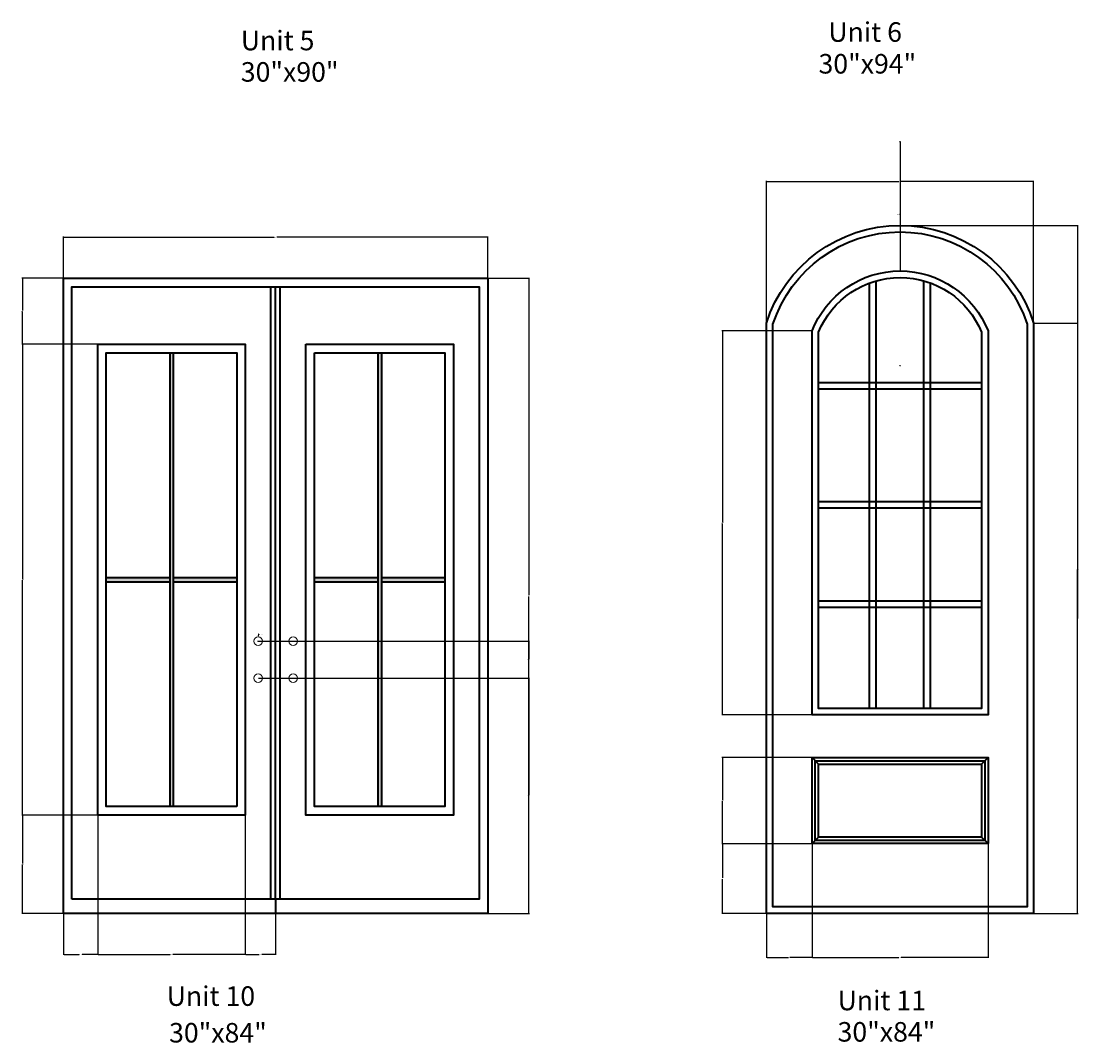
# Model space of a CAD drawing. Units: inches. Extents: x 1318 to 1980, y 617 to 1423.
# Tile 1 of 7: x 1318 to 1643, y 620 to 934. Entities that reach past the tile are written whole.
import ezdxf

# ---------------------------------------------------------------- set-up
doc = ezdxf.new("R2010")
doc.units = ezdxf.units.IN
doc.header["$MEASUREMENT"] = 0
for name, color, linetype, lineweight in [('A-ANNO-DIMS', 2, 'Continuous', 18), ('A-ANNO-TEXT', 7, 'Continuous', 25), ('A-DOOR', 4, 'Continuous', 35), ('A-DOOR-HDWR', 3, 'Continuous', 18), ('A-DOOR-PATT', 252, 'Continuous', 13)]:
    doc.layers.add(name, color=color, linetype=linetype, lineweight=lineweight)
doc.styles.get("Standard").update_dxf_attribs({"font": 'arial.ttf'})
doc.dimstyles.get("Standard").update_dxf_attribs({"dimtxt": 0.18, "dimasz": 0.18, "dimexe": 0.18, "dimexo": 0.0625, "dimgap": 0.09, "dimtad": 0, "dimtih": 1, "dimtoh": 1, "dimdec": 0, "dimzin": 0, "dimdsep": 46, "dimlunit": 3, "dimtxsty": 'Standard', "dimcen": 0.09, "dimadec": 0, "dimazin": 0, "dimtfac": 1, "dimtdec": 0, "dimtofl": 0, "dimtmove": 0, "dimatfit": 3, "dimfxl": 1, "dimtolj": 1, "dimtzin": 0, "dimarcsym": 0})

# ---------------------------------------------------------------- blocks, each defined once
blk = doc.blocks.new('*D76')
at = {"layer": 'A-ANNO-DIMS', "color": 0, "lineweight": -2, "transparency": 16777216}
for p, q in [((1390.63, 732.39), (1473.85, 732.39)), ((1473.67, 732.21), (1473.67, 696.45)), ((1473.67, 660.32), (1473.67, 696.09)), ((1395.97, 660.14), (1473.85, 660.14))]:
    blk.add_line(p, q, dxfattribs=at)
at = {"layer": 'A-ANNO-DIMS', "color": 0, "transparency": 16777216}
for points in [[(1473.64, 732.21), (1473.7, 732.21), (1473.67, 732.39)], [(1473.64, 660.32), (1473.7, 660.32), (1473.67, 660.14)]]:
    blk.add_solid(points, dxfattribs=at)
at = {"layer": 'Defpoints', "color": 0, "transparency": 16777216}
for p in [(1390.57, 732.39), (1473.67, 732.39), (1395.91, 660.14)]:
    blk.add_point(p, dxfattribs=at)
at = {"layer": 'A-ANNO-DIMS', "color": 0, "transparency": 16777216, "insert": (1473.67, 696.27), "char_height": 0.18, "attachment_point": 5}
blk.add_mtext('\\A1;72.24', dxfattribs=at)
blk = doc.blocks.new('*D77')
at = {"layer": 'A-ANNO-DIMS', "color": 0, "lineweight": -2, "transparency": 16777216}
for p, q in [((1390.63, 743.79), (1473.85, 743.79)), ((1473.67, 743.61), (1473.67, 738.27)), ((1473.67, 732.57), (1473.67, 737.91)), ((1390.63, 732.39), (1473.85, 732.39))]:
    blk.add_line(p, q, dxfattribs=at)
at = {"layer": 'A-ANNO-DIMS', "color": 0, "transparency": 16777216}
for points in [[(1473.64, 743.61), (1473.7, 743.61), (1473.67, 743.79)], [(1473.64, 732.57), (1473.7, 732.57), (1473.67, 732.39)]]:
    blk.add_solid(points, dxfattribs=at)
at = {"layer": 'Defpoints', "color": 0, "transparency": 16777216}
for p in [(1390.57, 743.79), (1473.67, 743.79), (1390.57, 732.39)]:
    blk.add_point(p, dxfattribs=at)
at = {"layer": 'A-ANNO-DIMS', "color": 0, "transparency": 16777216, "insert": (1473.67, 738.09), "char_height": 0.18, "attachment_point": 5}
blk.add_mtext('\\A1;11.405', dxfattribs=at)
blk = doc.blocks.new('*D78')
at = {"layer": 'A-ANNO-DIMS', "color": 0, "lineweight": -2, "transparency": 16777216}
for p, q in [((1330.76, 855.32), (1330.76, 868.04)), ((1330.94, 867.86), (1395.53, 867.86)), ((1460.89, 867.86), (1396.3, 867.86)), ((1461.07, 855.32), (1461.07, 868.04))]:
    blk.add_line(p, q, dxfattribs=at)
at = {"layer": 'A-ANNO-DIMS', "color": 0, "transparency": 16777216}
for points in [[(1330.94, 867.89), (1330.94, 867.83), (1330.76, 867.86)], [(1460.89, 867.89), (1460.89, 867.83), (1461.07, 867.86)]]:
    blk.add_solid(points, dxfattribs=at)
at = {"layer": 'Defpoints', "color": 0, "transparency": 16777216}
for p in [(1461.07, 867.86), (1330.76, 855.26), (1461.07, 855.26)]:
    blk.add_point(p, dxfattribs=at)
at = {"layer": 'A-ANNO-DIMS', "color": 0, "transparency": 16777216, "insert": (1395.91, 867.86), "char_height": 0.18, "attachment_point": 5}
blk.add_mtext('\\A1;130.3', dxfattribs=at)
blk = doc.blocks.new('*D79')
at = {"layer": 'A-ANNO-DIMS', "color": 0, "lineweight": -2, "transparency": 16777216}
for p, q in [((1461.13, 855.26), (1473.85, 855.26)), ((1473.67, 855.08), (1473.67, 757.88)), ((1473.67, 660.32), (1473.67, 757.52)), ((1461.13, 660.14), (1473.85, 660.14))]:
    blk.add_line(p, q, dxfattribs=at)
at = {"layer": 'A-ANNO-DIMS', "color": 0, "transparency": 16777216}
for points in [[(1473.64, 855.08), (1473.7, 855.08), (1473.67, 855.26)], [(1473.64, 660.32), (1473.7, 660.32), (1473.67, 660.14)]]:
    blk.add_solid(points, dxfattribs=at)
at = {"layer": 'Defpoints', "color": 0, "transparency": 16777216}
for p in [(1461.07, 855.26), (1473.67, 855.26), (1461.07, 660.14)]:
    blk.add_point(p, dxfattribs=at)
at = {"layer": 'A-ANNO-DIMS', "color": 0, "transparency": 16777216, "insert": (1473.67, 757.7), "char_height": 0.18, "attachment_point": 5}
blk.add_mtext('\\A1;195.1', dxfattribs=at)
blk = doc.blocks.new('*D80')
at = {"layer": 'A-ANNO-DIMS', "color": 0, "lineweight": -2, "transparency": 16777216}
for p, q in [((1341.29, 690.3), (1341.29, 647.36)), ((1330.76, 660.08), (1330.76, 647.36)), ((1330.94, 647.54), (1335.57, 647.54)), ((1341.11, 647.54), (1336.48, 647.54))]:
    blk.add_line(p, q, dxfattribs=at)
at = {"layer": 'A-ANNO-DIMS', "color": 0, "transparency": 16777216}
for points in [[(1330.94, 647.57), (1330.94, 647.51), (1330.76, 647.54)], [(1341.11, 647.57), (1341.11, 647.51), (1341.29, 647.54)]]:
    blk.add_solid(points, dxfattribs=at)
at = {"layer": 'Defpoints', "color": 0, "transparency": 16777216}
for p in [(1341.29, 690.36), (1330.76, 660.14), (1341.29, 647.54)]:
    blk.add_point(p, dxfattribs=at)
at = {"layer": 'A-ANNO-DIMS', "color": 0, "transparency": 16777216, "insert": (1336.02, 647.54), "char_height": 0.18, "attachment_point": 5}
blk.add_mtext('\\A1;10.532', dxfattribs=at)
blk = doc.blocks.new('*D81')
at = {"layer": 'A-ANNO-DIMS', "color": 0, "lineweight": -2, "transparency": 16777216}
for p, q in [((1341.29, 690.3), (1341.29, 647.36)), ((1386.61, 690.3), (1386.61, 647.36)), ((1341.47, 647.54), (1363.55, 647.54)), ((1386.43, 647.54), (1364.34, 647.54))]:
    blk.add_line(p, q, dxfattribs=at)
at = {"layer": 'A-ANNO-DIMS', "color": 0, "transparency": 16777216}
for points in [[(1341.47, 647.57), (1341.47, 647.51), (1341.29, 647.54)], [(1386.43, 647.57), (1386.43, 647.51), (1386.61, 647.54)]]:
    blk.add_solid(points, dxfattribs=at)
at = {"layer": 'Defpoints', "color": 0, "transparency": 16777216}
for p in [(1341.29, 690.36), (1386.61, 690.36), (1386.61, 647.54)]:
    blk.add_point(p, dxfattribs=at)
at = {"layer": 'A-ANNO-DIMS', "color": 0, "transparency": 16777216, "insert": (1363.95, 647.54), "char_height": 0.18, "attachment_point": 5}
blk.add_mtext('\\A1;45.32', dxfattribs=at)
blk = doc.blocks.new('*D82')
at = {"layer": 'A-ANNO-DIMS', "color": 0, "lineweight": -2, "transparency": 16777216}
for p, q in [((1386.61, 690.3), (1386.61, 647.36)), ((1395.91, 660.08), (1395.91, 647.36)), ((1386.79, 647.54), (1390.86, 647.54)), ((1395.73, 647.54), (1391.65, 647.54))]:
    blk.add_line(p, q, dxfattribs=at)
at = {"layer": 'A-ANNO-DIMS', "color": 0, "transparency": 16777216}
for points in [[(1386.79, 647.57), (1386.79, 647.51), (1386.61, 647.54)], [(1395.73, 647.57), (1395.73, 647.51), (1395.91, 647.54)]]:
    blk.add_solid(points, dxfattribs=at)
at = {"layer": 'Defpoints', "color": 0, "transparency": 16777216}
for p in [(1386.61, 690.36), (1395.91, 660.14), (1395.91, 647.54)]:
    blk.add_point(p, dxfattribs=at)
at = {"layer": 'A-ANNO-DIMS', "color": 0, "transparency": 16777216, "insert": (1391.26, 647.54), "char_height": 0.18, "attachment_point": 5}
blk.add_mtext('\\A1;9.305', dxfattribs=at)
blk = doc.blocks.new('*D83')
at = {"layer": 'A-ANNO-DIMS', "color": 0, "lineweight": -2, "transparency": 16777216}
for p, q in [((1341.23, 690.36), (1317.98, 690.36)), ((1318.16, 690.18), (1318.16, 675.43)), ((1318.16, 660.32), (1318.16, 675.07)), ((1330.69, 660.14), (1317.98, 660.14))]:
    blk.add_line(p, q, dxfattribs=at)
at = {"layer": 'A-ANNO-DIMS', "color": 0, "transparency": 16777216}
for points in [[(1318.13, 690.18), (1318.19, 690.18), (1318.16, 690.36)], [(1318.13, 660.32), (1318.19, 660.32), (1318.16, 660.14)]]:
    blk.add_solid(points, dxfattribs=at)
at = {"layer": 'Defpoints', "color": 0, "transparency": 16777216}
for p in [(1318.16, 690.36), (1341.29, 690.36), (1330.76, 660.14)]:
    blk.add_point(p, dxfattribs=at)
at = {"layer": 'A-ANNO-DIMS', "color": 0, "transparency": 16777216, "insert": (1318.16, 675.25), "char_height": 0.18, "attachment_point": 5}
blk.add_mtext('\\A1;30.214', dxfattribs=at)
blk = doc.blocks.new('*D84')
at = {"layer": 'A-ANNO-DIMS', "color": 0, "lineweight": -2, "transparency": 16777216}
for p, q in [((1341.23, 835), (1317.98, 835)), ((1318.16, 834.82), (1318.16, 762.86)), ((1318.16, 690.54), (1318.16, 762.5)), ((1341.23, 690.36), (1317.98, 690.36))]:
    blk.add_line(p, q, dxfattribs=at)
at = {"layer": 'A-ANNO-DIMS', "color": 0, "transparency": 16777216}
for points in [[(1318.13, 834.82), (1318.19, 834.82), (1318.16, 835)], [(1318.13, 690.54), (1318.19, 690.54), (1318.16, 690.36)]]:
    blk.add_solid(points, dxfattribs=at)
at = {"layer": 'Defpoints', "color": 0, "transparency": 16777216}
for p in [(1318.16, 835), (1341.29, 835), (1341.29, 690.36)]:
    blk.add_point(p, dxfattribs=at)
at = {"layer": 'A-ANNO-DIMS', "color": 0, "transparency": 16777216, "insert": (1318.16, 762.68), "char_height": 0.18, "attachment_point": 5}
blk.add_mtext('\\A1;144.64', dxfattribs=at)
blk = doc.blocks.new('*D85')
at = {"layer": 'A-ANNO-DIMS', "color": 0, "lineweight": -2, "transparency": 16777216}
for p, q in [((1330.69, 855.26), (1317.98, 855.26)), ((1318.16, 855.08), (1318.16, 845.31)), ((1318.16, 835.18), (1318.16, 844.95)), ((1341.23, 835), (1317.98, 835))]:
    blk.add_line(p, q, dxfattribs=at)
at = {"layer": 'A-ANNO-DIMS', "color": 0, "transparency": 16777216}
for points in [[(1318.13, 855.08), (1318.19, 855.08), (1318.16, 855.26)], [(1318.13, 835.18), (1318.19, 835.18), (1318.16, 835)]]:
    blk.add_solid(points, dxfattribs=at)
at = {"layer": 'Defpoints', "color": 0, "transparency": 16777216}
for p in [(1318.16, 855.26), (1330.76, 855.26), (1341.29, 835)]:
    blk.add_point(p, dxfattribs=at)
at = {"layer": 'A-ANNO-DIMS', "color": 0, "transparency": 16777216, "insert": (1318.16, 845.13), "char_height": 0.18, "attachment_point": 5}
blk.add_mtext('\\A1;20.257', dxfattribs=at)
blk = doc.blocks.new('*D86')
at = {"layer": 'A-ANNO-DIMS', "color": 0, "lineweight": -2, "transparency": 16777216}
for p, q in [((1546.65, 841.5), (1546.65, 885.18)), ((1546.83, 885), (1587.29, 885)), ((1628.53, 885), (1588.07, 885)), ((1628.71, 841.5), (1628.71, 885.18))]:
    blk.add_line(p, q, dxfattribs=at)
at = {"layer": 'A-ANNO-DIMS', "color": 0, "transparency": 16777216}
for points in [[(1546.83, 885.03), (1546.83, 884.97), (1546.65, 885)], [(1628.53, 885.03), (1628.53, 884.97), (1628.71, 885)]]:
    blk.add_solid(points, dxfattribs=at)
at = {"layer": 'Defpoints', "color": 0, "transparency": 16777216}
for p in [(1628.71, 885), (1546.65, 841.44), (1628.71, 841.44)]:
    blk.add_point(p, dxfattribs=at)
at = {"layer": 'A-ANNO-DIMS', "color": 0, "transparency": 16777216, "insert": (1587.68, 885), "char_height": 0.18, "attachment_point": 5}
blk.add_mtext('\\A1;82.07', dxfattribs=at)
blk = doc.blocks.new('*D87')
at = {"layer": 'A-ANNO-DIMS', "color": 0, "lineweight": -2, "transparency": 16777216}
for p, q in [((1628.78, 841.44), (1642.39, 841.44)), ((1642.21, 841.26), (1642.21, 750.97)), ((1642.21, 660.32), (1642.21, 750.61)), ((1628.78, 660.14), (1642.39, 660.14))]:
    blk.add_line(p, q, dxfattribs=at)
at = {"layer": 'A-ANNO-DIMS', "color": 0, "transparency": 16777216}
for points in [[(1642.18, 841.26), (1642.24, 841.26), (1642.21, 841.44)], [(1642.18, 660.32), (1642.24, 660.32), (1642.21, 660.14)]]:
    blk.add_solid(points, dxfattribs=at)
at = {"layer": 'Defpoints', "color": 0, "transparency": 16777216}
for p in [(1628.71, 841.44), (1642.21, 841.44), (1628.71, 660.14)]:
    blk.add_point(p, dxfattribs=at)
at = {"layer": 'A-ANNO-DIMS', "color": 0, "transparency": 16777216, "insert": (1642.21, 750.79), "char_height": 0.18, "attachment_point": 5}
blk.add_mtext('\\A1;181.3', dxfattribs=at)
blk = doc.blocks.new('*D88')
at = {"layer": 'A-ANNO-DIMS', "color": 0, "lineweight": -2, "transparency": 16777216}
for p, q in [((1587.74, 871.5), (1642.39, 871.5)), ((1642.21, 871.32), (1642.21, 766)), ((1642.21, 660.32), (1642.21, 765.64)), ((1546.71, 660.14), (1642.39, 660.14))]:
    blk.add_line(p, q, dxfattribs=at)
at = {"layer": 'A-ANNO-DIMS', "color": 0, "transparency": 16777216}
for points in [[(1642.18, 871.32), (1642.24, 871.32), (1642.21, 871.5)], [(1642.18, 660.32), (1642.24, 660.32), (1642.21, 660.14)]]:
    blk.add_solid(points, dxfattribs=at)
at = {"layer": 'Defpoints', "color": 0, "transparency": 16777216}
for p in [(1587.68, 871.5), (1642.21, 871.5), (1546.65, 660.14)]:
    blk.add_point(p, dxfattribs=at)
at = {"layer": 'A-ANNO-DIMS', "color": 0, "transparency": 16777216, "insert": (1642.21, 765.82), "char_height": 0.18, "attachment_point": 5}
blk.add_mtext('\\A1;211.35', dxfattribs=at)
blk = doc.blocks.new('*D89')
at = {"layer": 'A-ANNO-DIMS', "color": 0, "lineweight": -2, "transparency": 16777216}
for p, q in [((1560.65, 681.5), (1560.65, 646.46)), ((1546.65, 660.08), (1546.65, 646.46)), ((1546.83, 646.64), (1553.44, 646.64)), ((1560.47, 646.64), (1553.86, 646.64))]:
    blk.add_line(p, q, dxfattribs=at)
at = {"layer": 'A-ANNO-DIMS', "color": 0, "transparency": 16777216}
for points in [[(1546.83, 646.67), (1546.83, 646.61), (1546.65, 646.64)], [(1560.47, 646.67), (1560.47, 646.61), (1560.65, 646.64)]]:
    blk.add_solid(points, dxfattribs=at)
at = {"layer": 'Defpoints', "color": 0, "transparency": 16777216}
for p in [(1560.65, 681.56), (1546.65, 660.14), (1560.65, 646.64)]:
    blk.add_point(p, dxfattribs=at)
at = {"layer": 'A-ANNO-DIMS', "color": 0, "transparency": 16777216, "insert": (1553.65, 646.64), "char_height": 0.18, "attachment_point": 5}
blk.add_mtext('\\A1;14', dxfattribs=at)
blk = doc.blocks.new('*D90')
at = {"layer": 'A-ANNO-DIMS', "color": 0, "lineweight": -2, "transparency": 16777216}
for p, q in [((1560.65, 681.5), (1560.65, 646.46)), ((1614.71, 681.5), (1614.71, 646.46)), ((1560.83, 646.64), (1587.29, 646.64)), ((1614.53, 646.64), (1588.07, 646.64))]:
    blk.add_line(p, q, dxfattribs=at)
at = {"layer": 'A-ANNO-DIMS', "color": 0, "transparency": 16777216}
for points in [[(1560.83, 646.67), (1560.83, 646.61), (1560.65, 646.64)], [(1614.53, 646.67), (1614.53, 646.61), (1614.71, 646.64)]]:
    blk.add_solid(points, dxfattribs=at)
at = {"layer": 'Defpoints', "color": 0, "transparency": 16777216}
for p in [(1560.65, 681.56), (1614.71, 681.56), (1614.71, 646.64)]:
    blk.add_point(p, dxfattribs=at)
at = {"layer": 'A-ANNO-DIMS', "color": 0, "transparency": 16777216, "insert": (1587.68, 646.64), "char_height": 0.18, "attachment_point": 5}
blk.add_mtext('\\A1;54.07', dxfattribs=at)
blk = doc.blocks.new('*D91')
at = {"layer": 'A-ANNO-DIMS', "color": 0, "lineweight": -2, "transparency": 16777216}
for p, q in [((1560.59, 681.56), (1532.97, 681.56)), ((1533.15, 681.38), (1533.15, 671.04)), ((1533.15, 660.32), (1533.15, 670.67)), ((1546.59, 660.14), (1532.97, 660.14))]:
    blk.add_line(p, q, dxfattribs=at)
at = {"layer": 'A-ANNO-DIMS', "color": 0, "transparency": 16777216}
for points in [[(1533.12, 681.38), (1533.18, 681.38), (1533.15, 681.56)], [(1533.12, 660.32), (1533.18, 660.32), (1533.15, 660.14)]]:
    blk.add_solid(points, dxfattribs=at)
at = {"layer": 'Defpoints', "color": 0, "transparency": 16777216}
for p in [(1533.15, 681.56), (1560.65, 681.56), (1546.65, 660.14)]:
    blk.add_point(p, dxfattribs=at)
at = {"layer": 'A-ANNO-DIMS', "color": 0, "transparency": 16777216, "insert": (1533.15, 670.85), "char_height": 0.18, "attachment_point": 5}
blk.add_mtext('\\A1;21.418', dxfattribs=at)
blk = doc.blocks.new('*D92')
at = {"layer": 'A-ANNO-DIMS', "color": 0, "lineweight": -2, "transparency": 16777216}
for p, q in [((1560.59, 708.01), (1532.97, 708.01)), ((1533.15, 707.83), (1533.15, 694.97)), ((1533.15, 681.74), (1533.15, 694.61)), ((1560.59, 681.56), (1532.97, 681.56))]:
    blk.add_line(p, q, dxfattribs=at)
at = {"layer": 'A-ANNO-DIMS', "color": 0, "transparency": 16777216}
for points in [[(1533.12, 707.83), (1533.18, 707.83), (1533.15, 708.01)], [(1533.12, 681.74), (1533.18, 681.74), (1533.15, 681.56)]]:
    blk.add_solid(points, dxfattribs=at)
at = {"layer": 'Defpoints', "color": 0, "transparency": 16777216}
for p in [(1533.15, 708.01), (1560.65, 708.01), (1560.65, 681.56)]:
    blk.add_point(p, dxfattribs=at)
at = {"layer": 'A-ANNO-DIMS', "color": 0, "transparency": 16777216, "insert": (1533.15, 694.79), "char_height": 0.18, "attachment_point": 5}
blk.add_mtext('\\A1;26.45', dxfattribs=at)
blk = doc.blocks.new('*D93')
at = {"layer": 'A-ANNO-DIMS', "color": 0, "lineweight": -2, "transparency": 16777216}
for p, q in [((1560.59, 839.06), (1532.97, 839.06)), ((1533.15, 838.88), (1533.15, 780.27)), ((1533.15, 721.31), (1533.15, 779.91)), ((1560.59, 721.13), (1532.97, 721.13))]:
    blk.add_line(p, q, dxfattribs=at)
at = {"layer": 'A-ANNO-DIMS', "color": 0, "transparency": 16777216}
for points in [[(1533.12, 838.88), (1533.18, 838.88), (1533.15, 839.06)], [(1533.12, 721.31), (1533.18, 721.31), (1533.15, 721.13)]]:
    blk.add_solid(points, dxfattribs=at)
at = {"layer": 'Defpoints', "color": 0, "transparency": 16777216}
for p in [(1533.15, 839.06), (1560.65, 839.06), (1560.65, 721.13)]:
    blk.add_point(p, dxfattribs=at)
at = {"layer": 'A-ANNO-DIMS', "color": 0, "transparency": 16777216, "insert": (1533.15, 780.09), "char_height": 0.18, "attachment_point": 5}
blk.add_mtext('\\A1;117.93', dxfattribs=at)
blk = doc.blocks.new('*D115')
at = {"layer": 'A-ANNO-DIMS', "color": 0, "lineweight": -2, "transparency": 16777216}
for p, q in [((1390.57, 743.7), (1390.57, 743.88)), ((1390.62, 745.92), (1390.6, 745.3)), ((1390.8, 745.92), (1390.62, 745.92)), ((1390.48, 743.79), (1390.66, 743.79))]:
    blk.add_line(p, q, dxfattribs=at)
at = {"layer": 'A-ANNO-DIMS', "color": 0, "transparency": 16777216}
blk.add_solid([(1390.57, 745.3), (1390.63, 745.3), (1390.6, 745.12)], dxfattribs=at)
at = {"layer": 'Defpoints', "color": 0, "transparency": 16777216}
for p in [(1390.6, 745.12), (1390.53, 742.46)]:
    blk.add_point(p, dxfattribs=at)
at = {"layer": 'A-ANNO-DIMS', "color": 0, "transparency": 16777216, "insert": (1391.41, 745.92), "char_height": 0.18, "attachment_point": 5}
blk.add_mtext('\\A1;4X ∅2.66', dxfattribs=at)
blk = doc.blocks.new('*D116')
at = {"layer": 'A-ANNO-DIMS', "color": 0, "lineweight": -2, "transparency": 16777216}
for p, q in [((1587.5, 897.32), (1587.68, 897.32)), ((1587.68, 897.32), (1587.68, 871.68)), ((1587.59, 828.46), (1587.77, 828.46)), ((1587.68, 828.37), (1587.68, 828.55))]:
    blk.add_line(p, q, dxfattribs=at)
at = {"layer": 'A-ANNO-DIMS', "color": 0, "transparency": 16777216}
blk.add_solid([(1587.71, 871.68), (1587.65, 871.68), (1587.68, 871.5)], dxfattribs=at)
at = {"layer": 'Defpoints', "color": 0, "transparency": 16777216}
for p in [(1587.68, 871.5), (1587.68, 828.46)]:
    blk.add_point(p, dxfattribs=at)
at = {"layer": 'A-ANNO-DIMS', "color": 0, "transparency": 16777216, "insert": (1587.02, 897.32), "char_height": 0.18, "attachment_point": 5}
blk.add_mtext('\\A1;R43.04', dxfattribs=at)
blk = doc.blocks.new('*D117')
at = {"layer": 'A-ANNO-DIMS', "color": 0, "lineweight": -2, "transparency": 16777216}
for p, q in [((1587.5, 874.92), (1587.68, 874.92)), ((1587.68, 874.92), (1587.68, 857.68)), ((1587.59, 828.46), (1587.77, 828.46)), ((1587.68, 828.37), (1587.68, 828.55))]:
    blk.add_line(p, q, dxfattribs=at)
at = {"layer": 'A-ANNO-DIMS', "color": 0, "transparency": 16777216}
blk.add_solid([(1587.71, 857.68), (1587.65, 857.68), (1587.68, 857.5)], dxfattribs=at)
at = {"layer": 'Defpoints', "color": 0, "transparency": 16777216}
for p in [(1587.68, 857.5), (1587.68, 828.46)]:
    blk.add_point(p, dxfattribs=at)
at = {"layer": 'A-ANNO-DIMS', "color": 0, "transparency": 16777216, "insert": (1587.02, 874.92), "char_height": 0.18, "attachment_point": 5}
blk.add_mtext('\\A1;R29.04', dxfattribs=at)

msp = doc.modelspace()

# ---------------------------------------------------------------- hatches: boundary and pattern name
at = {"layer": 'A-DOOR-PATT'}
h = msp.add_hatch(color=256, dxfattribs=at)
h.dxf.hatch_style = 1
h.paths.add_polyline_path([(1364.5134, 762.0215), (1383.9731, 762.0215), (1383.9731, 763.338), (1364.5134, 763.338)])
h.paths.add_polyline_path([(1364.5134, 832.3675), (1363.4292, 832.3675), (1363.4292, 692.9919), (1364.5134, 692.9919)])
h.paths.add_polyline_path([(1343.9224, 763.338), (1343.9224, 762.0215), (1363.4292, 762.0215), (1363.4292, 763.338)])
h.paths.add_polyline_path([(1447.9005, 762.0215), (1447.9005, 763.338), (1428.4408, 763.338), (1428.4408, 762.0215)])
h.paths.add_polyline_path([(1427.3566, 762.0215), (1427.3566, 763.338), (1407.8498, 763.338), (1407.8498, 762.0215)])
h.paths.add_polyline_path([(1427.3566, 692.9919), (1428.4408, 692.9919), (1428.4408, 832.3675), (1427.3566, 832.3675)])

# ---------------------------------------------------------------- linework, layer by layer
at = {"layer": 'A-DOOR'}
for p, q in [((1580.3374, 723.1263), (1580.3374, 854.4796)), ((1595.0329, 723.1263), (1595.0329, 854.4771)), ((1394.5054, 664.4806), (1394.5054, 852.6245)), ((1395.9114, 664.4806), (1395.9114, 852.6245)), ((1397.3175, 664.4806), (1397.3175, 852.6245)), ((1578.3374, 723.1263), (1578.3374, 853.8302)), ((1597.0329, 723.1263), (1597.0329, 853.827)), ((1363.4292, 832.3675), (1363.4292, 692.9919)), ((1364.5134, 832.3675), (1364.5134, 692.9919)), ((1427.3566, 832.3675), (1427.3566, 692.9919)), ((1428.4408, 832.3675), (1428.4408, 692.9919)), ((1562.6475, 823.2404), (1612.7141, 823.2404)), ((1562.6475, 821.2404), (1612.7141, 821.2404)), ((1562.6475, 786.7141), (1612.7141, 786.7141)), ((1562.6475, 784.7141), (1612.7141, 784.7141)), ((1343.9224, 763.338), (1363.4292, 763.338)), ((1364.5134, 763.338), (1383.9731, 763.338)), ((1407.8498, 763.338), (1427.3566, 763.338)), ((1428.4408, 763.338), (1447.9005, 763.338)), ((1343.9224, 762.0215), (1363.4292, 762.0215)), ((1364.5134, 762.0215), (1383.9731, 762.0215)), ((1407.8498, 762.0215), (1427.3566, 762.0215)), ((1428.4408, 762.0215), (1447.9005, 762.0215)), ((1562.6475, 756.1843), (1612.7141, 756.1843)), ((1562.6475, 754.1843), (1612.7141, 754.1843)), ((1560.6475, 708.0115), (1562.6475, 706.0115)), ((1562.6475, 706.0115), (1562.6475, 706.0115)), ((1614.7141, 708.0115), (1612.7141, 706.0115)), ((1562.6475, 683.5627), (1560.6475, 681.5627)), ((1612.7141, 683.5627), (1614.7141, 681.5627)), ((1395.9114, 664.4806), (1395.9114, 660.1449))]:
    msp.add_line(p, q, dxfattribs=at)
for points in [[(1628.7141, 841.4384), (1628.7141, 660.1449), (1546.6475, 660.1449), (1546.6475, 841.4384, -0.73251551)], [(1626.7141, 841.1259), (1626.7141, 662.1449), (1548.6475, 662.1449), (1548.6475, 841.1259, -0.72681718)], [(1614.7141, 839.0588), (1614.7141, 721.1263), (1560.6475, 721.1263), (1560.6475, 839.0588, -0.68201543)], [(1612.7141, 838.6737), (1612.7141, 723.1263), (1562.6475, 723.1263), (1562.6475, 838.6737, -0.67199378)]]:
    msp.add_lwpolyline(points, format="xyb", close=True, dxfattribs=at)
for points in [[(1330.757, 855.2576), (1461.0659, 855.2576), (1461.0659, 660.1449), (1330.757, 660.1449)], [(1333.3901, 664.4806), (1333.3901, 852.6245), (1458.4328, 852.6245), (1458.4328, 664.4806)], [(1386.6062, 690.3589), (1341.2893, 690.3589), (1341.2893, 835.0006), (1386.6062, 835.0006)], [(1405.2167, 835.0006), (1450.5336, 835.0006), (1450.5336, 690.3589), (1405.2167, 690.3589)], [(1383.9731, 692.9919), (1343.9224, 692.9919), (1343.9224, 832.3675), (1383.9731, 832.3675)], [(1407.8498, 832.3675), (1447.9005, 832.3675), (1447.9005, 692.9919), (1407.8498, 692.9919)], [(1560.6475, 708.0115), (1614.7141, 708.0115), (1614.7141, 681.5627), (1560.6475, 681.5627)], [(1561.6475, 707.0115), (1613.7141, 707.0115), (1613.7141, 682.5627), (1561.6475, 682.5627)], [(1562.6475, 706.0115), (1612.7141, 706.0115), (1612.7141, 683.5627), (1562.6475, 683.5627)]]:
    msp.add_lwpolyline(points, close=True, dxfattribs=at)
at = {"layer": 'A-DOOR-HDWR'}
for centre in [(1390.5654, 743.7922), (1401.29, 743.7922), (1390.5654, 732.3871), (1401.29, 732.3871)]:
    msp.add_circle(centre, 1.3278, dxfattribs=at)

# ---------------------------------------------------------------- texts
at = {"layer": 'A-ANNO-TEXT'}
for s, p in [('Unit 6', (1565.6638, 927.9049)), ('Unit 5', (1385.2363, 925.2927)), ('30"x94"', (1562.6428, 918.1503)), ('30"x90"', (1385.2363, 915.6542)), ('Unit 10', (1362.479, 631.7324)), ('Unit 11', (1568.4986, 630.3875)), ('30"x84"', (1568.4986, 620.749)), ('30"x84"', (1363.2076, 620.4749))]:
    msp.add_text(s, height=6, dxfattribs=at).set_placement(p)

# ---------------------------------------------------------------- dimensions: what is measured, and where the dimension line sits
at = {"layer": 'A-ANNO-DIMS'}
for mpoint, picture, middle in [((1587.68, 871.4959), '*D116', (1587.02, 897.3183)), ((1587.68, 857.4959), '*D117', (1587.02, 874.9183))]:
    dim = msp.add_radius_dim(center=(1587.6808, 828.4587), mpoint=mpoint, dimstyle='Standard', override={"dimdec": 2, "dimlfac": 1, "dimrnd": 0, "dimzin": 0, "dimdsep": 46, "dimlunit": 2}, dxfattribs=at)
    dim.commit()
    dim.dimension.update_dxf_attribs({"geometry": picture, "text_midpoint": middle, "dimtype": 164})
for base, p1, p2, override, picture, middle in [((1628.7141, 884.9959), (1546.6475, 841.4384), (1628.7141, 841.4384), {"dimdec": 2, "dimlfac": 1, "dimrnd": 0, "dimzin": 0, "dimdsep": 46, "dimlunit": 2}, '*D86', (1587.6808, 884.9959)), ((1461.0659, 867.8576), (1330.757, 855.2576), (1461.0659, 855.2576), {"dimdec": 1, "dimlfac": 1, "dimrnd": 0, "dimzin": 0, "dimdsep": 46, "dimlunit": 2}, '*D78', (1395.9114, 867.8576)), ((1341.2893, 647.5449), (1330.757, 660.1449), (1341.2893, 690.3589), {"dimdec": 3, "dimlfac": 1, "dimrnd": 0, "dimzin": 0, "dimdsep": 46, "dimlunit": 2}, '*D80', (1336.0231, 647.5449)), ((1386.6062, 647.5449), (1341.2893, 690.3589), (1386.6062, 690.3589), {"dimdec": 2, "dimlfac": 1, "dimrnd": 0, "dimzin": 0, "dimdsep": 46, "dimlunit": 2}, '*D81', (1363.9477, 647.5449)), ((1395.9114, 647.5449), (1386.6062, 690.3589), (1395.9114, 660.1449), {"dimdec": 3, "dimlfac": 1, "dimrnd": 0, "dimzin": 0, "dimdsep": 46, "dimlunit": 2}, '*D82', (1391.2588, 647.5449)), ((1560.6475, 646.6449), (1546.6475, 660.1449), (1560.6475, 681.5627), {"dimdec": 0, "dimlfac": 1, "dimrnd": 0, "dimzin": 0, "dimdsep": 46, "dimlunit": 2}, '*D89', (1553.6475, 646.6449)), ((1614.7141, 646.6449), (1560.6475, 681.5627), (1614.7141, 681.5627), {"dimdec": 2, "dimlfac": 1, "dimrnd": 0, "dimzin": 0, "dimdsep": 46, "dimlunit": 2}, '*D90', (1587.6808, 646.6449))]:
    dim = msp.add_linear_dim(base=base, p1=p1, p2=p2, dimstyle='Standard', override=override, dxfattribs=at)
    dim.commit()
    dim.dimension.update_dxf_attribs({"geometry": picture, "text_midpoint": middle})
for base, p1, p2, override, picture, middle in [((1642.2141, 871.4959), (1546.6475, 660.1449), (1587.6808, 871.4959), {"dimdec": 2, "dimlfac": 1, "dimrnd": 0, "dimzin": 0, "dimdsep": 46, "dimlunit": 2}, '*D88', (1642.2141, 765.8204)), ((1318.157, 855.2576), (1341.2893, 835.0006), (1330.757, 855.2576), {"dimdec": 3, "dimlfac": 1, "dimrnd": 0, "dimzin": 0, "dimdsep": 46, "dimlunit": 2}, '*D85', (1318.157, 845.1291)), ((1473.6659, 855.2576), (1461.0659, 660.1449), (1461.0659, 855.2576), {"dimdec": 1, "dimlfac": 1, "dimrnd": 0, "dimzin": 0, "dimdsep": 46, "dimlunit": 2}, '*D79', (1473.6659, 757.7012)), ((1642.2141, 841.4384), (1628.7141, 660.1449), (1628.7141, 841.4384), {"dimdec": 1, "dimlfac": 1, "dimrnd": 0, "dimzin": 0, "dimdsep": 46, "dimlunit": 2}, '*D87', (1642.2141, 750.7916)), ((1533.1475, 839.0588), (1560.6475, 721.1263), (1560.6475, 839.0588), {"dimdec": 2, "dimlfac": 1, "dimrnd": 0, "dimzin": 0, "dimdsep": 46, "dimlunit": 2}, '*D93', (1533.1475, 780.0926)), ((1318.157, 835.0006), (1341.2893, 690.3589), (1341.2893, 835.0006), {"dimdec": 2, "dimlfac": 1, "dimrnd": 0, "dimzin": 0, "dimdsep": 46, "dimlunit": 2}, '*D84', (1318.157, 762.6797)), ((1473.6659, 743.7922), (1390.5654, 732.3871), (1390.5654, 743.7922), {"dimdec": 3, "dimlfac": 1, "dimrnd": 0, "dimzin": 0, "dimdsep": 46, "dimlunit": 2}, '*D77', (1473.6659, 738.0896)), ((1473.6659, 732.3871), (1395.9114, 660.1449), (1390.5654, 732.3871), {"dimdec": 2, "dimlfac": 1, "dimrnd": 0, "dimzin": 0, "dimdsep": 46, "dimlunit": 2}, '*D76', (1473.6659, 696.266)), ((1533.1475, 708.0115), (1560.6475, 681.5627), (1560.6475, 708.0115), {"dimdec": 2, "dimlfac": 1, "dimrnd": 0, "dimzin": 0, "dimdsep": 46, "dimlunit": 2}, '*D92', (1533.1475, 694.7871)), ((1318.157, 690.3589), (1330.757, 660.1449), (1341.2893, 690.3589), {"dimdec": 3, "dimlfac": 1, "dimrnd": 0, "dimzin": 0, "dimdsep": 46, "dimlunit": 2}, '*D83', (1318.157, 675.2519)), ((1533.1475, 681.5627), (1546.6475, 660.1449), (1560.6475, 681.5627), {"dimdec": 3, "dimlfac": 1, "dimrnd": 0, "dimzin": 0, "dimdsep": 46, "dimlunit": 2}, '*D91', (1533.1475, 670.8538))]:
    dim = msp.add_linear_dim(base=base, p1=p1, p2=p2, angle=90, dimstyle='Standard', override=override, dxfattribs=at)
    dim.commit()
    dim.dimension.update_dxf_attribs({"geometry": picture, "text_midpoint": middle})
dim = msp.add_diameter_dim_2p(p1=(1390.5316, 742.4648), p2=(1390.5992, 745.1195), text='4X <>', dimstyle='Standard', override={"dimdec": 2, "dimlfac": 1, "dimrnd": 0, "dimzin": 0, "dimdsep": 46, "dimlunit": 2}, dxfattribs=at)
dim.commit()
dim.dimension.update_dxf_attribs({"geometry": '*D115', "text_midpoint": (1391.4134, 745.9159), "dimtype": 163})

doc.saveas('drawing.dxf')
